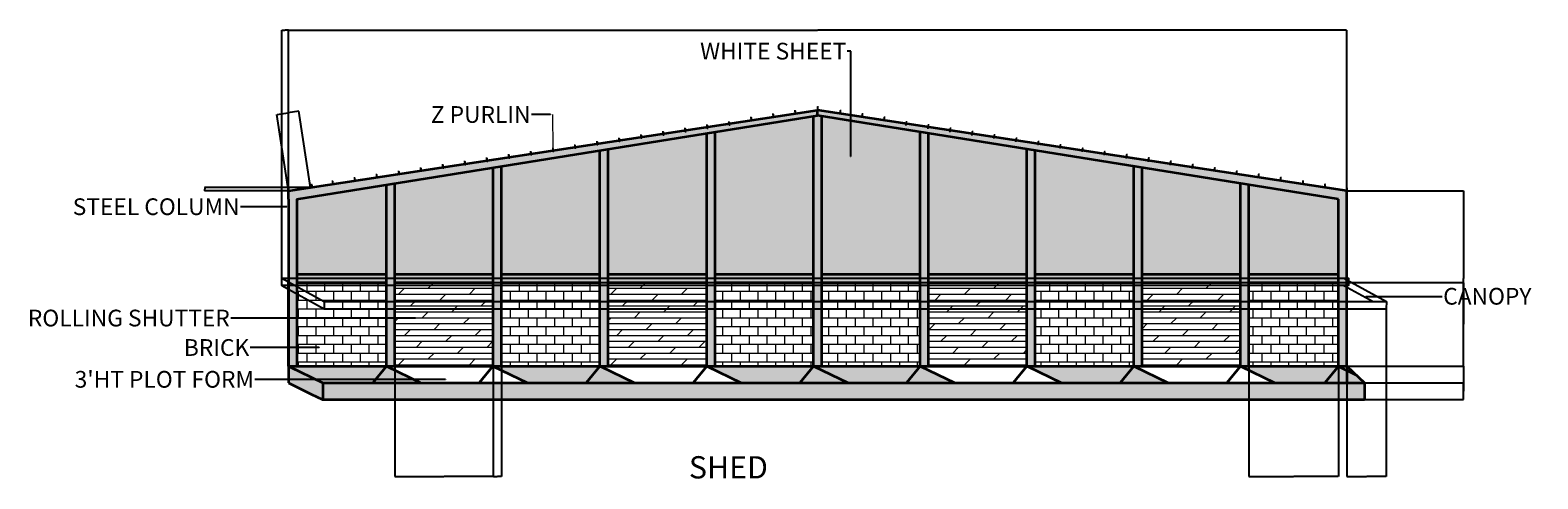
# Model space of a CAD drawing. Units: inches. Extents: x 1136 to 4385, y 1177 to 2144.
import ezdxf
from ezdxf import colors
from ezdxf.entities.mleader import LeaderData, LeaderLine
from ezdxf.math import Vec2, Vec3

# ---------------------------------------------------------------- set-up
doc = ezdxf.new("R2010")
doc.units = ezdxf.units.IN
for name, color, linetype, lineweight in [('A-ANNO-DIMS', 2, 'Continuous', 18), ('A-ANNO-TEXT', 7, 'Continuous', 18), ('A-DOOR-PATT', 8, 'Continuous', 13), ('A-FLOR-PLAT', 7, 'Continuous', 35), ('A-WALL-PATT', 8, 'Continuous', 13), ('S-BEAM', 7, 'Continuous', 35), ('S-COLS', 7, 'Continuous', 35), ('S-ROOF-PURL', 7, 'Continuous', 25)]:
    doc.layers.add(name, color=color, linetype=linetype, lineweight=lineweight)
for name, color, linetype, lineweight, true_color in [('A-FLOR-PATT', 30, 'Continuous', 13, 0xf26722), ('A-ROOF-CNPY', 240, 'Continuous', 25, 0xed1f24), ('A-WALL-CLAD-PATT', 7, 'Continuous', 13, 0xffffff), ('S-FRAM-PATT', 252, 'Continuous', 13, 0x939598)]:
    doc.layers.add(name, color=color, linetype=linetype, lineweight=lineweight, true_color=true_color)
doc.styles.get("Standard").update_dxf_attribs({"font": 'arial.ttf'})
doc.dimstyles.get("Standard").update_dxf_attribs({"dimtxt": 0.18, "dimasz": 0.18, "dimexe": 0.18, "dimexo": 0.0625, "dimgap": 0.09, "dimtad": 0, "dimtih": 1, "dimtoh": 1, "dimdec": 4, "dimzin": 0, "dimdsep": 46, "dimtxsty": 'Standard', "dimcen": 0.09, "dimadec": 0, "dimazin": 0, "dimtfac": 1, "dimtdec": 4, "dimtofl": 0, "dimtmove": 0, "dimatfit": 3, "dimfxl": 1, "dimtolj": 1, "dimtzin": 0, "dimarcsym": 0})

# ---------------------------------------------------------------- blocks, each defined once
blk = doc.blocks.new('PURLIN-Z-6IN')
blk.add_lwpolyline([(0, 6), (2, 6), (2, 0), (4, 0)])
blk = doc.blocks.new('*D2')
at = {"layer": 'A-ANNO-DIMS', "color": 0, "lineweight": -2, "transparency": 16777216}
for p, q in [((1742.7, 1810.9), (1743.7, 1810.9)), ((1742.7, 1804.9), (1743.7, 1804.9)), ((1743.5, 1810.7), (1743.5, 1808.1)), ((1743.5, 1805.1), (1743.5, 1807.7))]:
    blk.add_line(p, q, dxfattribs=at)
at = {"layer": 'A-ANNO-DIMS', "color": 0, "transparency": 16777216}
for points in [[(1743.5, 1810.7), (1743.6, 1810.7), (1743.5, 1810.9)], [(1743.5, 1805.1), (1743.6, 1805.1), (1743.5, 1804.9)]]:
    blk.add_solid(points, dxfattribs=at)
at = {"layer": 'Defpoints', "color": 0, "transparency": 16777216}
for p in [(1742.6, 1810.9), (1742.6, 1804.9), (1743.5, 1810.9)]:
    blk.add_point(p, dxfattribs=at)
at = {"layer": 'A-ANNO-DIMS', "color": 0, "transparency": 16777216, "insert": (1743.5, 1807.9), "char_height": 0.18, "attachment_point": 5}
blk.add_mtext('\\A1;Z PURLIN 6 TYP.', dxfattribs=at)
blk = doc.blocks.new('*D3')
at = {"layer": 'A-ANNO-DIMS', "color": 0, "lineweight": -2, "transparency": 16777216}
for p, q in [((1738.6, 1804.8), (1738.6, 1803.8)), ((1738.8, 1804), (1740.2, 1804)), ((1742.5, 1804), (1741.1, 1804)), ((1742.6, 1804.8), (1742.6, 1803.8))]:
    blk.add_line(p, q, dxfattribs=at)
at = {"layer": 'A-ANNO-DIMS', "color": 0, "transparency": 16777216}
for points in [[(1738.8, 1804), (1738.8, 1804), (1738.6, 1804)], [(1742.5, 1804), (1742.5, 1804), (1742.6, 1804)]]:
    blk.add_solid(points, dxfattribs=at)
at = {"layer": 'Defpoints', "color": 0, "transparency": 16777216}
for p in [(1738.6, 1804.9), (1742.6, 1804.9), (1742.6, 1804)]:
    blk.add_point(p, dxfattribs=at)
at = {"layer": 'A-ANNO-DIMS', "color": 0, "transparency": 16777216, "insert": (1740.6, 1804), "char_height": 0.18, "attachment_point": 5}
blk.add_mtext('\\A1;4 TYP.', dxfattribs=at)
blk = doc.blocks.new('*D4')
at = {"layer": 'A-ANNO-DIMS', "color": 0, "lineweight": -2, "transparency": 16777216}
for p, q in [((1693.184241, 1797.715563), (1693.184241, 2143.833063)), ((1693.364241, 2143.653063), (2832.824241, 2143.653063)), ((3973.004241, 2143.653063), (2833.544241, 2143.653063)), ((3973.184241, 1797.715563), (3973.184241, 2143.833063))]:
    blk.add_line(p, q, dxfattribs=at)
at = {"layer": 'A-ANNO-DIMS', "color": 0, "transparency": 16777216}
for points in [[(1693.364241, 2143.683063), (1693.364241, 2143.623063), (1693.184241, 2143.653063)], [(3973.004241, 2143.683063), (3973.004241, 2143.623063), (3973.184241, 2143.653063)]]:
    blk.add_solid(points, dxfattribs=at)
at = {"layer": 'Defpoints', "color": 0, "transparency": 16777216}
for p in [(3973.184241, 2143.653063), (1693.184241, 1797.653063), (3973.184241, 1797.653063)]:
    blk.add_point(p, dxfattribs=at)
at = {"layer": 'A-ANNO-DIMS', "color": 0, "transparency": 16777216, "insert": (2833.184241, 2143.653063), "char_height": 0.18, "attachment_point": 5}
blk.add_mtext('\\A1;2280', dxfattribs=at)
blk = doc.blocks.new('*D5')
at = {"layer": 'A-ANNO-DIMS', "color": 0, "lineweight": -2, "transparency": 16777216}
for p, q in [((3973.2, 1797.7), (4224.9, 1797.7)), ((4224.7, 1797.5), (4224.7, 1608.8)), ((4224.7, 1419.8), (4224.7, 1608.5)), ((3973.2, 1419.7), (4224.9, 1419.7))]:
    blk.add_line(p, q, dxfattribs=at)
at = {"layer": 'A-ANNO-DIMS', "color": 0, "transparency": 16777216}
for points in [[(4224.7, 1797.5), (4224.8, 1797.5), (4224.7, 1797.7)], [(4224.7, 1419.8), (4224.8, 1419.8), (4224.7, 1419.7)]]:
    blk.add_solid(points, dxfattribs=at)
at = {"layer": 'Defpoints', "color": 0, "transparency": 16777216}
for p in [(3973.2, 1797.7), (4224.7, 1797.7), (3973.2, 1419.7)]:
    blk.add_point(p, dxfattribs=at)
at = {"layer": 'A-ANNO-DIMS', "color": 0, "transparency": 16777216, "insert": (4224.7, 1608.7), "char_height": 0.18, "attachment_point": 5}
blk.add_mtext('\\A1;378', dxfattribs=at)
blk = doc.blocks.new('*D6')
at = {"layer": 'A-ANNO-DIMS', "color": 0, "lineweight": -2, "transparency": 16777216}
for p, q in [((4058.5, 1543.4), (4058.5, 1181.5)), ((3973.2, 1419.6), (3973.2, 1181.5)), ((3973.4, 1181.7), (4015.5, 1181.7)), ((4058.3, 1181.7), (4016.2, 1181.7))]:
    blk.add_line(p, q, dxfattribs=at)
at = {"layer": 'A-ANNO-DIMS', "color": 0, "transparency": 16777216}
for points in [[(3973.4, 1181.7), (3973.4, 1181.6), (3973.2, 1181.7)], [(4058.3, 1181.7), (4058.3, 1181.6), (4058.5, 1181.7)]]:
    blk.add_solid(points, dxfattribs=at)
at = {"layer": 'Defpoints', "color": 0, "transparency": 16777216}
for p in [(4058.5, 1543.5), (3973.2, 1419.7), (3973.2, 1181.7)]:
    blk.add_point(p, dxfattribs=at)
at = {"layer": 'A-ANNO-DIMS', "color": 0, "transparency": 16777216, "insert": (4015.8, 1181.7), "char_height": 0.18, "attachment_point": 5}
blk.add_mtext('\\A1;85.3', dxfattribs=at)
blk = doc.blocks.new('*D7')
at = {"layer": 'A-ANNO-DIMS', "color": 0, "lineweight": -2, "transparency": 16777216}
for p, q in [((1678.6, 1609.2), (1678.6, 2143.8)), ((1678.8, 2143.7), (1685.5, 2143.7)), ((1693, 2143.7), (1686.2, 2143.7)), ((1693.2, 1797.7), (1693.2, 2143.8))]:
    blk.add_line(p, q, dxfattribs=at)
at = {"layer": 'A-ANNO-DIMS', "color": 0, "transparency": 16777216}
for points in [[(1678.8, 2143.7), (1678.8, 2143.6), (1678.6, 2143.7)], [(1693, 2143.7), (1693, 2143.6), (1693.2, 2143.7)]]:
    blk.add_solid(points, dxfattribs=at)
at = {"layer": 'Defpoints', "color": 0, "transparency": 16777216}
for p in [(1693.2, 2143.7), (1693.2, 1797.7), (1678.6, 1609.1)]:
    blk.add_point(p, dxfattribs=at)
at = {"layer": 'A-ANNO-DIMS', "color": 0, "transparency": 16777216, "insert": (1685.9, 2143.7), "char_height": 0.18, "attachment_point": 5}
blk.add_mtext('\\A1;14.61', dxfattribs=at)
blk = doc.blocks.new('*D8')
at = {"layer": 'A-ANNO-DIMS', "color": 0, "lineweight": -2, "transparency": 16777216}
for p, q in [((4011.4, 1383.7), (4224.9, 1383.7)), ((4224.7, 1383.5), (4224.7, 1365.8)), ((4224.7, 1347.8), (4224.7, 1365.5)), ((4011.4, 1347.7), (4224.9, 1347.7))]:
    blk.add_line(p, q, dxfattribs=at)
at = {"layer": 'A-ANNO-DIMS', "color": 0, "transparency": 16777216}
for points in [[(4224.7, 1383.5), (4224.8, 1383.5), (4224.7, 1383.7)], [(4224.7, 1347.8), (4224.8, 1347.8), (4224.7, 1347.7)]]:
    blk.add_solid(points, dxfattribs=at)
at = {"layer": 'Defpoints', "color": 0, "transparency": 16777216}
for p in [(4011.3, 1383.7), (4224.7, 1383.7), (4011.3, 1347.7)]:
    blk.add_point(p, dxfattribs=at)
at = {"layer": 'A-ANNO-DIMS', "color": 0, "transparency": 16777216, "insert": (4224.7, 1365.7), "char_height": 0.18, "attachment_point": 5}
blk.add_mtext('\\A1;36', dxfattribs=at)
blk = doc.blocks.new('*D9')
at = {"layer": 'A-ANNO-DIMS', "color": 0, "lineweight": -2, "transparency": 16777216}
for p, q in [((1922.2, 1599.7), (4224.9, 1599.7)), ((4224.7, 1599.5), (4224.7, 1509.8)), ((4224.7, 1419.8), (4224.7, 1509.5)), ((1922.2, 1419.7), (4224.9, 1419.7))]:
    blk.add_line(p, q, dxfattribs=at)
at = {"layer": 'A-ANNO-DIMS', "color": 0, "transparency": 16777216}
for points in [[(4224.7, 1599.5), (4224.8, 1599.5), (4224.7, 1599.7)], [(4224.7, 1419.8), (4224.8, 1419.8), (4224.7, 1419.7)]]:
    blk.add_solid(points, dxfattribs=at)
at = {"layer": 'Defpoints', "color": 0, "transparency": 16777216}
for p in [(1922.2, 1599.7), (4224.7, 1599.7), (1922.2, 1419.7)]:
    blk.add_point(p, dxfattribs=at)
at = {"layer": 'A-ANNO-DIMS', "color": 0, "transparency": 16777216, "insert": (4224.7, 1509.7), "char_height": 0.18, "attachment_point": 5}
blk.add_mtext('\\A1;180', dxfattribs=at)
blk = doc.blocks.new('*D10')
at = {"layer": 'A-ANNO-DIMS', "color": 0, "lineweight": -2, "transparency": 16777216}
for p, q in [((1922.2, 1419.6), (1922.2, 1181.5)), ((2134.2, 1419.6), (2134.2, 1181.5)), ((1922.4, 1181.7), (2027.9, 1181.7)), ((2134, 1181.7), (2028.5, 1181.7))]:
    blk.add_line(p, q, dxfattribs=at)
at = {"layer": 'A-ANNO-DIMS', "color": 0, "transparency": 16777216}
for points in [[(1922.4, 1181.7), (1922.4, 1181.6), (1922.2, 1181.7)], [(2134, 1181.7), (2134, 1181.6), (2134.2, 1181.7)]]:
    blk.add_solid(points, dxfattribs=at)
at = {"layer": 'Defpoints', "color": 0, "transparency": 16777216}
for p in [(1922.2, 1419.7), (2134.2, 1419.7), (2134.2, 1181.7)]:
    blk.add_point(p, dxfattribs=at)
at = {"layer": 'A-ANNO-DIMS', "color": 0, "transparency": 16777216, "insert": (2028.2, 1181.7), "char_height": 0.18, "attachment_point": 5}
blk.add_mtext('\\A1;212', dxfattribs=at)
blk = doc.blocks.new('*D11')
at = {"layer": 'A-ANNO-DIMS', "color": 0, "lineweight": -2, "transparency": 16777216}
for p, q in [((2134.2, 1419.6), (2134.2, 1181.5)), ((2152.2, 1419.6), (2152.2, 1181.5)), ((2134.4, 1181.7), (2143, 1181.7)), ((2152, 1181.7), (2143.4, 1181.7))]:
    blk.add_line(p, q, dxfattribs=at)
at = {"layer": 'A-ANNO-DIMS', "color": 0, "transparency": 16777216}
for points in [[(2134.4, 1181.7), (2134.4, 1181.6), (2134.2, 1181.7)], [(2152, 1181.7), (2152, 1181.6), (2152.2, 1181.7)]]:
    blk.add_solid(points, dxfattribs=at)
at = {"layer": 'Defpoints', "color": 0, "transparency": 16777216}
for p in [(2134.2, 1419.7), (2152.2, 1419.7), (2152.2, 1181.7)]:
    blk.add_point(p, dxfattribs=at)
at = {"layer": 'A-ANNO-DIMS', "color": 0, "transparency": 16777216, "insert": (2143.2, 1181.7), "char_height": 0.18, "attachment_point": 5}
blk.add_mtext('\\A1;18', dxfattribs=at)
blk = doc.blocks.new('*D12')
at = {"layer": 'A-ANNO-DIMS', "color": 0, "lineweight": -2, "transparency": 16777216}
for p, q in [((3762.2, 1419.6), (3762.2, 1181.5)), ((3955.2, 1419.6), (3955.2, 1181.5)), ((3762.4, 1181.7), (3858.4, 1181.7)), ((3955, 1181.7), (3859, 1181.7))]:
    blk.add_line(p, q, dxfattribs=at)
at = {"layer": 'A-ANNO-DIMS', "color": 0, "transparency": 16777216}
for points in [[(3762.4, 1181.7), (3762.4, 1181.6), (3762.2, 1181.7)], [(3955, 1181.7), (3955, 1181.6), (3955.2, 1181.7)]]:
    blk.add_solid(points, dxfattribs=at)
at = {"layer": 'Defpoints', "color": 0, "transparency": 16777216}
for p in [(3762.2, 1419.7), (3955.2, 1419.7), (3955.2, 1181.7)]:
    blk.add_point(p, dxfattribs=at)
at = {"layer": 'A-ANNO-DIMS', "color": 0, "transparency": 16777216, "insert": (3858.7, 1181.7), "char_height": 0.18, "attachment_point": 5}
blk.add_mtext('\\A1;193', dxfattribs=at)
blk = doc.blocks.new('*D13')
at = {"layer": 'A-ANNO-DIMS', "color": 0, "lineweight": -2, "transparency": 16777216}
for p, q in [((1693.2, 1797.7), (1668.1, 1961.9)), ((1668.3, 1961.8), (1691.6, 1965.3)), ((1715.4, 1969), (1692.1, 1965.4)), ((1740.6, 1805), (1715.6, 1969.2))]:
    blk.add_line(p, q, dxfattribs=at)
at = {"layer": 'A-ANNO-DIMS', "color": 0, "transparency": 16777216}
for points in [[(1668.3, 1961.8), (1668.3, 1961.8), (1668.1, 1961.8)], [(1715.4, 1969), (1715.4, 1968.9), (1715.6, 1969)]]:
    blk.add_solid(points, dxfattribs=at)
at = {"layer": 'Defpoints', "color": 0, "transparency": 16777216}
for p in [(1715.6, 1969), (1693.2, 1797.7), (1740.6, 1804.9)]:
    blk.add_point(p, dxfattribs=at)
at = {"layer": 'A-ANNO-DIMS', "color": 0, "transparency": 16777216, "insert": (1691.9, 1965.4), "char_height": 0.18, "attachment_point": 5}
blk.add_mtext('\\A1;48', dxfattribs=at)
blk = doc.blocks.new('*D14')
at = {"layer": 'A-ANNO-DIMS', "color": 0, "lineweight": -2, "transparency": 16777216}
for p, q in [((1740.6, 1804.9), (1512.4, 1804.9)), ((1693.1, 1797.7), (1512.4, 1797.7)), ((1512.6, 1804.7), (1512.6, 1801.5)), ((1512.6, 1797.8), (1512.6, 1801.1))]:
    blk.add_line(p, q, dxfattribs=at)
at = {"layer": 'A-ANNO-DIMS', "color": 0, "transparency": 16777216}
for points in [[(1512.5, 1804.7), (1512.6, 1804.7), (1512.6, 1804.9)], [(1512.5, 1797.8), (1512.6, 1797.8), (1512.6, 1797.7)]]:
    blk.add_solid(points, dxfattribs=at)
at = {"layer": 'Defpoints', "color": 0, "transparency": 16777216}
for p in [(1512.6, 1804.9), (1693.2, 1797.7), (1740.6, 1804.9)]:
    blk.add_point(p, dxfattribs=at)
at = {"layer": 'A-ANNO-DIMS', "color": 0, "transparency": 16777216, "insert": (1512.6, 1801.3), "char_height": 0.18, "attachment_point": 5}
blk.add_mtext('\\A1;7.242', dxfattribs=at)
blk = doc.blocks.new('*D15')
at = {"layer": 'A-ANNO-DIMS', "color": 0, "lineweight": -2, "transparency": 16777216}
for p, q in [((3973.2, 1419.7), (4224.9, 1419.7)), ((4224.7, 1419.5), (4224.7, 1383.8)), ((4224.7, 1347.8), (4224.7, 1383.5)), ((4011.4, 1347.7), (4224.9, 1347.7))]:
    blk.add_line(p, q, dxfattribs=at)
at = {"layer": 'A-ANNO-DIMS', "color": 0, "transparency": 16777216}
for points in [[(4224.7, 1419.5), (4224.8, 1419.5), (4224.7, 1419.7)], [(4224.7, 1347.8), (4224.8, 1347.8), (4224.7, 1347.7)]]:
    blk.add_solid(points, dxfattribs=at)
at = {"layer": 'Defpoints', "color": 0, "transparency": 16777216}
for p in [(3973.2, 1419.7), (4011.3, 1347.7), (4224.7, 1347.7)]:
    blk.add_point(p, dxfattribs=at)
at = {"layer": 'A-ANNO-DIMS', "color": 0, "transparency": 16777216, "insert": (4224.7, 1383.7), "char_height": 0.18, "attachment_point": 5}
blk.add_mtext('\\A1;72', dxfattribs=at)

msp = doc.modelspace()

# ---------------------------------------------------------------- hatches: boundary and pattern name
at = {"layer": 'A-DOOR-PATT'}
h = msp.add_hatch(dxfattribs=at)
h.set_pattern_fill('DOLMIT', color=256, scale=2)
h.paths.add_polyline_path([(2134.1842, 1599.6531), (1922.1842, 1599.6531), (1922.1842, 1419.6531), (2134.1842, 1419.6531)])
h.paths.add_polyline_path([(2594.1842, 1599.6531), (2382.1842, 1599.6531), (2382.1842, 1419.6531), (2594.1842, 1419.6531)])
h.paths.add_polyline_path([(3284.1842, 1599.6531), (3072.1842, 1599.6531), (3072.1842, 1419.6531), (3284.1842, 1419.6531)])
h.paths.add_polyline_path([(3744.1842, 1599.6531), (3532.1842, 1599.6531), (3532.1842, 1419.6531), (3744.1842, 1419.6531)])
at = {"layer": 'A-FLOR-PATT'}
h = msp.add_hatch(color=256, dxfattribs=at)
h.dxf.hatch_style = 1
h.paths.add_polyline_path([(1904.1842, 1419.6531), (1693.1842, 1419.6531), (1767.3542, 1383.6531), (1874.7817, 1383.6531)])
h.paths.add_polyline_path([(4011.303, 1383.6531), (1767.3542, 1383.6531), (1767.3542, 1347.6531), (4011.303, 1347.6531)])
h.paths.add_polyline_path([(1767.3542, 1383.6531), (1693.1842, 1419.6531), (1693.1842, 1383.6531), (1742.1622, 1359.5845), (1766.442, 1347.6531), (1767.3542, 1347.6531)])
h.paths.add_polyline_path([(3992.81, 1401.1182), (3973.1842, 1410.644), (3973.1842, 1383.6531), (4011.303, 1383.6531)])
h.paths.add_polyline_path([(3973.1842, 1419.6531), (3955.5362, 1419.6531), (3955.277, 1419.3357), (3992.81, 1401.1182)])
h.paths.add_polyline_path([(3973.1842, 1410.644), (3955.277, 1419.3357), (3926.1337, 1383.6531), (3973.1842, 1383.6531)])
h.paths.add_polyline_path([(3955.1842, 1419.2221), (3955.1842, 1419.3807), (3954.6231, 1419.6531), (3744.4245, 1419.6531), (3818.5945, 1383.6531), (3926.1337, 1383.6531)])
h.paths.add_polyline_path([(3514.4245, 1419.6531), (3514.1842, 1419.6531), (3484.7817, 1383.6531), (3588.5945, 1383.6531)])
h.paths.add_polyline_path([(3514.1842, 1419.6531), (3284.4245, 1419.6531), (3358.5945, 1383.6531), (3484.7817, 1383.6531)])
h.paths.add_polyline_path([(3054.4245, 1419.6531), (3054.1842, 1419.6531), (3024.7817, 1383.6531), (3128.5945, 1383.6531)])
h.paths.add_polyline_path([(3054.1842, 1419.6531), (2824.4245, 1419.6531), (2898.5945, 1383.6531), (3024.7817, 1383.6531)])
h.paths.add_polyline_path([(2824.4245, 1419.6531), (2824.1842, 1419.6531), (2794.7817, 1383.6531), (2898.5945, 1383.6531)])
h.paths.add_polyline_path([(2364.1842, 1419.6531), (2133.5344, 1419.6531), (2207.7043, 1383.6531), (2334.7817, 1383.6531)])
h.paths.add_polyline_path([(2364.4245, 1419.6531), (2364.1842, 1419.6531), (2334.7817, 1383.6531), (2438.5945, 1383.6531)])
h.paths.add_polyline_path([(2824.1842, 1419.6531), (2594.4245, 1419.6531), (2668.5945, 1383.6531), (2794.7817, 1383.6531)])
h.paths.add_polyline_path([(1904.1842, 1419.6531), (1874.7817, 1383.6531), (1978.3542, 1383.6531)])
at = {"layer": 'A-WALL-CLAD-PATT'}
h = msp.add_hatch(color=256, dxfattribs=at)
h.dxf.hatch_style = 1
h.paths.add_polyline_path([(1904.1842, 1810.6156), (1711.1842, 1779.6531), (1711.1842, 1617.6531), (1904.1842, 1617.6531)])
h.paths.add_polyline_path([(2134.1842, 1847.514), (1922.1842, 1813.5033), (1922.1842, 1617.6531), (2134.1842, 1617.6531)])
h.paths.add_polyline_path([(2364.1842, 1884.4124), (2152.1842, 1850.4017), (2152.1842, 1617.6531), (2364.1842, 1617.6531)])
h.paths.add_polyline_path([(2594.1842, 1921.3108), (2382.1842, 1887.3001), (2382.1842, 1617.6531), (2594.1842, 1617.6531)])
h.paths.add_polyline_path([(2824.1842, 1958.2092), (2612.1842, 1924.1985), (2612.1842, 1617.6531), (2824.1842, 1617.6531)])
h.paths.add_polyline_path([(3054.1842, 1924.1985), (2842.1842, 1958.2092), (2842.1842, 1617.6531), (3054.1842, 1617.6531)])
h.paths.add_polyline_path([(3284.1842, 1887.3001), (3072.1842, 1921.3108), (3072.1842, 1617.6531), (3284.1842, 1617.6531)])
h.paths.add_polyline_path([(3514.1842, 1850.4017), (3302.1842, 1884.4124), (3302.1842, 1617.6531), (3514.1842, 1617.6531)])
h.paths.add_polyline_path([(3744.1842, 1813.5033), (3532.1842, 1847.514), (3532.1842, 1617.6531), (3744.1842, 1617.6531)])
h.paths.add_polyline_path([(3955.1842, 1779.6531), (3762.1842, 1810.6156), (3762.1842, 1617.6531), (3955.1842, 1617.6531)])
at = {"layer": 'A-WALL-PATT'}
h = msp.add_hatch(dxfattribs=at)
h.set_pattern_fill('BRICK', color=256, scale=3)
h.paths.add_polyline_path([(1904.1842, 1599.6531), (1711.1842, 1599.6531), (1711.1842, 1419.6531), (1904.1842, 1419.6531)])
h.paths.add_polyline_path([(2364.1842, 1599.6531), (2152.1842, 1599.6531), (2152.1842, 1419.6531), (2364.1842, 1419.6531)])
h.paths.add_polyline_path([(2824.1842, 1599.6531), (2612.1842, 1599.6531), (2612.1842, 1419.6531), (2824.1842, 1419.6531)])
h.paths.add_polyline_path([(3054.1842, 1599.6531), (2842.1842, 1599.6531), (2842.1842, 1419.6531), (3054.1842, 1419.6531)])
h.paths.add_polyline_path([(3514.1842, 1599.6531), (3302.1842, 1599.6531), (3302.1842, 1419.6531), (3514.1842, 1419.6531)])
h.paths.add_polyline_path([(3955.1842, 1599.6531), (3762.1842, 1599.6531), (3762.1842, 1419.6531), (3955.1842, 1419.6531)])
at = {"layer": 'S-FRAM-PATT'}
h = msp.add_hatch(color=256, dxfattribs=at)
h.dxf.hatch_style = 1
h.paths.add_polyline_path([(1711.1842, 1779.6531), (2833.1842, 1959.6531), (2833.1842, 1971.6531), (1693.1842, 1797.6531), (1693.1842, 1779.6531), (1693.1842, 1419.6531), (1711.1842, 1419.6531)])
h.paths.add_polyline_path([(1904.1842, 1617.6531), (1711.1842, 1617.6531), (1711.1842, 1599.6531), (1904.1842, 1599.6531)], flags=17)
h.paths.add_polyline_path([(2134.1842, 1617.6531), (1922.1842, 1617.6531), (1922.1842, 1599.6531), (2134.1842, 1599.6531)], flags=17)
h = msp.add_hatch(color=256, dxfattribs=at)
h.dxf.hatch_style = 1
h.paths.add_polyline_path([(1922.1842, 1813.5033), (1904.1842, 1810.6156), (1904.1842, 1419.6531), (1922.1842, 1419.6531)])
h.paths.add_polyline_path([(2152.1842, 1850.4017), (2134.1842, 1847.514), (2134.1842, 1419.6531), (2152.1842, 1419.6531)])
h.paths.add_polyline_path([(2382.1842, 1887.3001), (2364.1842, 1884.4124), (2364.1842, 1419.6531), (2382.1842, 1419.6531)])
h.paths.add_polyline_path([(2364.1842, 1617.6531), (2152.1842, 1617.6531), (2152.1842, 1599.6531), (2364.1842, 1599.6531)])
h.paths.add_polyline_path([(2594.1842, 1617.6531), (2382.1842, 1617.6531), (2382.1842, 1599.6531), (2594.1842, 1599.6531)])
h.paths.add_polyline_path([(2612.1842, 1924.1985), (2594.1842, 1921.3108), (2594.1842, 1419.6531), (2612.1842, 1419.6531)])
h.paths.add_polyline_path([(2824.1842, 1617.6531), (2612.1842, 1617.6531), (2612.1842, 1599.6531), (2824.1842, 1599.6531)])
h.paths.add_polyline_path([(2842.1842, 1958.2092), (2833.1842, 1959.6531), (2824.1842, 1958.2092), (2824.1842, 1419.6531), (2842.1842, 1419.6531)])
h.paths.add_polyline_path([(3054.1842, 1617.6531), (2842.1842, 1617.6531), (2842.1842, 1599.6531), (3054.1842, 1599.6531)], flags=17)
h.paths.add_polyline_path([(3072.1842, 1921.3108), (3054.1842, 1924.1985), (3054.1842, 1419.6531), (3072.1842, 1419.6531)], flags=17)
h.paths.add_polyline_path([(3284.1842, 1617.6531), (3072.1842, 1617.6531), (3072.1842, 1599.6531), (3284.1842, 1599.6531)], flags=17)
h.paths.add_polyline_path([(3302.1842, 1884.4124), (3284.1842, 1887.3001), (3284.1842, 1419.6531), (3302.1842, 1419.6531)], flags=17)
h.paths.add_polyline_path([(3514.1842, 1617.6531), (3302.1842, 1617.6531), (3302.1842, 1599.6531), (3514.1842, 1599.6531)], flags=17)
h.paths.add_polyline_path([(3532.1842, 1847.514), (3514.1842, 1850.4017), (3514.1842, 1419.6531), (3532.1842, 1419.6531)], flags=17)
h.paths.add_polyline_path([(3955.1842, 1617.6531), (3762.1842, 1617.6531), (3762.1842, 1599.6531), (3955.1842, 1599.6531)], flags=17)
h.paths.add_polyline_path([(3973.1842, 1797.6531), (2833.1842, 1971.6531), (2833.1842, 1959.6531), (2842.1842, 1958.2092), (3955.1842, 1779.6531), (3955.1842, 1419.6531), (3973.1842, 1419.6531)])
h = msp.add_hatch(color=256, dxfattribs=at)
h.dxf.hatch_style = 1
h.paths.add_polyline_path([(3762.1842, 1810.6156), (3744.1842, 1813.5033), (3744.1842, 1419.6531), (3762.1842, 1419.6531)])
h.paths.add_polyline_path([(3744.1842, 1617.6531), (3532.1842, 1617.6531), (3532.1842, 1599.6531), (3744.1842, 1599.6531)])

# ---------------------------------------------------------------- linework, layer by layer
at = {"layer": 'A-ANNO-TEXT'}
msp.add_line((2261.8285, 1961.7238), (2262.8285, 1888.9845), dxfattribs=at)
at = {"layer": 'A-FLOR-PLAT'}
for p, q in [((1693.1842, 1419.6531), (3973.1842, 1419.6531)), ((1693.1842, 1419.6531), (1693.1842, 1383.6531)), ((1693.1842, 1419.6531), (1767.3542, 1383.6531)), ((1693.1842, 1419.6531), (1725.6025, 1403.9987)), ((1904.1842, 1419.6531), (1874.7817, 1383.6531)), ((1904.1842, 1419.6531), (1978.3542, 1383.6531)), ((2133.5344, 1419.6531), (2104.1318, 1383.6531)), ((2133.5344, 1419.6531), (2207.7043, 1383.6531)), ((2364.1842, 1419.6531), (2334.7817, 1383.6531)), ((2364.4245, 1419.6531), (2438.5945, 1383.6531)), ((2594.1842, 1419.6531), (2564.7817, 1383.6531)), ((2594.4245, 1419.6531), (2668.5945, 1383.6531)), ((2824.1842, 1419.6531), (2794.7817, 1383.6531)), ((2824.4245, 1419.6531), (2898.5945, 1383.6531)), ((3054.1842, 1419.6531), (3024.7817, 1383.6531)), ((3054.4245, 1419.6531), (3128.5945, 1383.6531)), ((3284.1842, 1419.6531), (3254.7817, 1383.6531)), ((3284.4245, 1419.6531), (3358.5945, 1383.6531)), ((3514.1842, 1419.6531), (3484.7817, 1383.6531)), ((3514.4245, 1419.6531), (3588.5945, 1383.6531)), ((3744.1842, 1419.6531), (3714.7817, 1383.6531)), ((3744.4245, 1419.6531), (3818.5945, 1383.6531)), ((3955.5362, 1419.6531), (3926.1337, 1383.6531)), ((3954.6231, 1419.6531), (3992.81, 1401.1182)), ((3973.1842, 1419.6531), (4011.303, 1383.6531)), ((3973.1842, 1410.644), (3973.1842, 1383.6531)), ((1693.1842, 1383.6531), (1742.1622, 1359.5845)), ((1767.3542, 1383.6531), (4011.303, 1383.6531)), ((1767.3542, 1383.6531), (1767.3542, 1347.6531)), ((4011.303, 1383.6531), (4011.303, 1347.6531)), ((1742.1622, 1359.5845), (1766.442, 1347.6531)), ((1766.442, 1347.6531), (4011.303, 1347.6531))]:
    msp.add_line(p, q, dxfattribs=at)
at = {"layer": 'A-ROOF-CNPY'}
for p, q in [((1678.5734, 1609.1255), (1770.081, 1559.1366)), ((1678.5734, 1593.4739), (1770.0695, 1543.4913)), ((3967.2276, 1609.1255), (4058.7352, 1559.1366)), ((3967.2276, 1593.4739), (4030.084, 1559.1366)), ((1770.0695, 1543.4913), (4058.4842, 1543.4913)), ((1770.081, 1559.1366), (4058.7352, 1559.1366)), ((1770.081, 1559.1366), (1770.081, 1543.4913)), ((4058.7352, 1559.1366), (4058.4842, 1543.4913))]:
    msp.add_line(p, q, dxfattribs=at)
msp.add_lwpolyline([(1678.5734, 1609.1255), (3977.0566, 1609.1255), (3977.0566, 1593.4739), (1678.5734, 1593.4739)], close=True, dxfattribs=at)
at = {"layer": 'S-BEAM'}
for p, q in [((1693.1842, 1797.6531), (2833.1842, 1971.6531)), ((1711.1842, 1779.6531), (2833.1842, 1959.6531)), ((2833.1842, 1959.6531), (2833.1842, 1971.6531)), ((3973.1842, 1797.6531), (2833.1842, 1971.6531)), ((2833.1842, 1959.6531), (2833.1842, 1971.6531)), ((3955.1842, 1779.6531), (2833.1842, 1959.6531)), ((1693.1842, 1779.6531), (1693.1842, 1797.6531)), ((1711.1842, 1617.6531), (1904.1842, 1617.6531)), ((1711.1842, 1599.6531), (1904.1842, 1599.6531)), ((1922.1842, 1617.6531), (2134.1842, 1617.6531)), ((1922.1842, 1599.6531), (2134.1842, 1599.6531)), ((2152.1842, 1617.6531), (2364.1842, 1617.6531)), ((2152.1842, 1599.6531), (2364.1842, 1599.6531)), ((2382.1842, 1617.6531), (2594.1842, 1617.6531)), ((2382.1842, 1599.6531), (2594.1842, 1599.6531)), ((2612.1842, 1617.6531), (2824.1842, 1617.6531)), ((2612.1842, 1599.6531), (2824.1842, 1599.6531)), ((2842.1842, 1617.6531), (3054.1842, 1617.6531)), ((2842.1842, 1599.6531), (3054.1842, 1599.6531)), ((3072.1842, 1617.6531), (3284.1842, 1617.6531)), ((3072.1842, 1599.6531), (3284.1842, 1599.6531)), ((3302.1842, 1617.6531), (3514.1842, 1617.6531)), ((3302.1842, 1599.6531), (3514.1842, 1599.6531)), ((3532.1842, 1617.6531), (3744.1842, 1617.6531)), ((3532.1842, 1599.6531), (3744.1842, 1599.6531)), ((3762.1842, 1617.6531), (3955.1842, 1617.6531)), ((3762.1842, 1599.6531), (3955.1842, 1599.6531))]:
    msp.add_line(p, q, dxfattribs=at)
at = {"layer": 'S-COLS'}
for p, q in [((2824.1842, 1419.6531), (2824.1842, 1958.2092)), ((2842.1842, 1419.6531), (2842.1842, 1958.2092)), ((2594.1842, 1419.6531), (2594.1842, 1921.3108)), ((2612.1842, 1419.6531), (2612.1842, 1924.1985)), ((3054.1842, 1419.6531), (3054.1842, 1924.1985)), ((3072.1842, 1419.6531), (3072.1842, 1921.3108)), ((2364.1842, 1419.6531), (2364.1842, 1884.4124)), ((2382.1842, 1419.6531), (2382.1842, 1887.3001)), ((3284.1842, 1419.6531), (3284.1842, 1887.3001)), ((3302.1842, 1419.6531), (3302.1842, 1884.4124)), ((2134.1842, 1419.6531), (2134.1842, 1847.514)), ((2152.1842, 1419.6531), (2152.1842, 1850.4017)), ((3514.1842, 1419.6531), (3514.1842, 1850.4017)), ((3532.1842, 1419.6531), (3532.1842, 1847.514)), ((1904.1842, 1419.6531), (1904.1842, 1810.6156)), ((1922.1842, 1419.6531), (1922.1842, 1813.5033)), ((3744.1842, 1419.6531), (3744.1842, 1813.5033)), ((3762.1842, 1419.6531), (3762.1842, 1810.6156)), ((3973.1842, 1419.6531), (3973.1842, 1797.6531)), ((1693.1842, 1779.6531), (1693.1842, 1419.6531)), ((1711.1842, 1779.6531), (1711.1842, 1419.6531)), ((3955.1842, 1419.6531), (3955.1842, 1779.6531)), ((1693.1842, 1419.6531), (1693.1842, 1599.6531))]:
    msp.add_line(p, q, dxfattribs=at)

# ---------------------------------------------------------------- block references
at = {"layer": 'S-ROOF-PURL'}
for p in [(2687.6439, 1949.7442), (2735.0943, 1956.9867), (2782.5448, 1964.2291), (2831.184, 1971.653), (2450.7096, 1911.4283), (2498.18, 1918.5392), (2545.6503, 1925.6502), (2593.1207, 1932.7611), (2640.6119, 1939.733), (2260.8282, 1882.9845), (2308.2986, 1890.0954), (2355.7689, 1897.2064), (2403.2393, 1904.3173), (2023.4765, 1847.4297), (2070.9468, 1854.5406), (2118.4172, 1861.6516), (2165.8875, 1868.7625), (2213.3579, 1875.8735), (1833.5354, 1819.3803), (1880.9859, 1826.6228), (1928.5358, 1833.2078), (1976.0061, 1840.3187), (1691.184, 1797.653), (1738.6345, 1804.8954), (1786.0849, 1812.1379)]:
    msp.add_blockref('PURLIN-Z-6IN', p, dxfattribs=at)
at = {"layer": 'S-ROOF-PURL', "extrusion": (0, 0, -1), "zscale": -1}
for p in [(-2835.1845, 1971.653), (-2883.8237, 1964.2291), (-2931.2742, 1956.9867), (-2978.7246, 1949.7442), (-3025.7566, 1939.733), (-3073.2478, 1932.7611), (-3120.7181, 1925.6502), (-3168.1885, 1918.5392), (-3215.6588, 1911.4283), (-3263.1292, 1904.3173), (-3310.5996, 1897.2064), (-3358.0699, 1890.0954), (-3405.5403, 1882.9845), (-3453.0106, 1875.8735), (-3500.481, 1868.7625), (-3547.9513, 1861.6516), (-3595.4217, 1854.5406), (-3642.892, 1847.4297), (-3690.3624, 1840.3187), (-3737.8327, 1833.2078), (-3785.3826, 1826.6228), (-3832.8331, 1819.3803), (-3880.2835, 1812.1379), (-3927.734, 1804.8954), (-3975.1845, 1797.653)]:
    msp.add_blockref('PURLIN-Z-6IN', p, dxfattribs=at)

# ---------------------------------------------------------------- texts
at = {"layer": 'A-ANNO-TEXT', "insert": (2555.7451, 1225.5789), "char_height": 48, "attachment_point": 1}
msp.add_mtext_dynamic_manual_height_columns('SHED', width=465.265352, gutter_width=12.5, heights=[0], dxfattribs=at)

# ---------------------------------------------------------------- dimensions: what is measured, and where the dimension line sits
at = {"layer": 'A-ANNO-DIMS'}
for base, p1, p2, override, picture, middle in [((1693.1842, 2143.6531), (1678.5734, 1609.1255), (1693.1842, 1797.6531), {"dimdec": 2, "dimlfac": 1, "dimrnd": 0, "dimzin": 0, "dimdsep": 46, "dimlunit": 2}, '*D7', (1685.8788, 2143.6531)), ((3973.1842, 2143.6531), (1693.1842, 1797.6531), (3973.1842, 1797.6531), {"dimdec": 0, "dimlfac": 1, "dimrnd": 0, "dimzin": 0, "dimdsep": 46, "dimlunit": 2}, '*D4', (2833.1842, 2143.6531)), ((3973.1842, 1181.6531), (4058.4842, 1543.4913), (3973.1842, 1419.6531), {"dimdec": 1, "dimlfac": 1, "dimrnd": 0, "dimzin": 0, "dimdsep": 46, "dimlunit": 2}, '*D6', (4015.8342, 1181.6531)), ((2134.1842, 1181.6531), (1922.1842, 1419.6531), (2134.1842, 1419.6531), {"dimdec": 0, "dimlfac": 1, "dimrnd": 0, "dimzin": 0, "dimdsep": 46, "dimlunit": 2}, '*D10', (2028.1842, 1181.6531)), ((2152.1842, 1181.6531), (2134.1842, 1419.6531), (2152.1842, 1419.6531), {"dimdec": 0, "dimlfac": 1, "dimrnd": 0, "dimzin": 0, "dimdsep": 46, "dimlunit": 2}, '*D11', (2143.1842, 1181.6531)), ((3955.1842, 1181.6531), (3762.1842, 1419.6531), (3955.1842, 1419.6531), {"dimdec": 0, "dimlfac": 1, "dimrnd": 0, "dimzin": 0, "dimdsep": 46, "dimlunit": 2}, '*D12', (3858.6842, 1181.6531))]:
    dim = msp.add_linear_dim(base=base, p1=p1, p2=p2, dimstyle='Standard', override=override, dxfattribs=at)
    dim.commit()
    dim.dimension.update_dxf_attribs({"geometry": picture, "text_midpoint": middle})
for base, p1, p2, angle, override, picture, middle in [((1715.5879, 1968.995), (1693.1842, 1797.6531), (1740.6347, 1804.8955), 8.6781689, {"dimdec": 0, "dimlfac": 1, "dimrnd": 0, "dimzin": 0, "dimdsep": 46, "dimlunit": 2}, '*D13', (1691.8627, 1965.3738)), ((1512.5734, 1804.8955), (1693.1842, 1797.6531), (1740.6347, 1804.8955), 90, {"dimdec": 3, "dimlfac": 1, "dimrnd": 0, "dimzin": 0, "dimdsep": 46, "dimlunit": 2}, '*D14', (1512.5734, 1801.2743)), ((4224.7352, 1797.6531), (3973.1842, 1419.6531), (3973.1842, 1797.6531), 90, {"dimdec": 0, "dimlfac": 1, "dimrnd": 0, "dimzin": 0, "dimdsep": 46, "dimlunit": 2}, '*D5', (4224.7352, 1608.6531)), ((4224.7352, 1599.6531), (1922.1842, 1419.6531), (1922.1842, 1599.6531), 90, {"dimdec": 0, "dimlfac": 1, "dimrnd": 0, "dimzin": 0, "dimdsep": 46, "dimlunit": 2}, '*D9', (4224.7352, 1509.6531)), ((4224.7352, 1347.6531), (3973.1842, 1419.6531), (4011.303, 1347.6531), 90, {"dimdec": 0, "dimlfac": 1, "dimrnd": 0, "dimzin": 0, "dimdsep": 46, "dimlunit": 2}, '*D15', (4224.7352, 1383.6531)), ((4224.7352, 1383.6531), (4011.303, 1347.6531), (4011.303, 1383.6531), 90, {"dimdec": 0, "dimlfac": 1, "dimrnd": 0, "dimzin": 0, "dimdsep": 46, "dimlunit": 2}, '*D8', (4224.7352, 1365.6531))]:
    dim = msp.add_linear_dim(base=base, p1=p1, p2=p2, angle=angle, dimstyle='Standard', override=override, dxfattribs=at)
    dim.commit()
    dim.dimension.update_dxf_attribs({"geometry": picture, "text_midpoint": middle})
dim = msp.add_linear_dim(base=(1742.6347, 1803.9955), p1=(1738.6347, 1804.8955), p2=(1742.6347, 1804.8955), text='<> TYP.', dimstyle='Standard', override={"dimdec": 0, "dimlfac": 1, "dimrnd": 0, "dimzin": 0, "dimdsep": 46, "dimlunit": 2}, dxfattribs=at)
dim.commit()
dim.dimension.update_dxf_attribs({"geometry": '*D3', "text_midpoint": (1740.6347, 1803.9955)})
dim = msp.add_linear_dim(base=(1743.5347, 1810.8955), p1=(1742.6347, 1804.8955), p2=(1742.6347, 1810.8955), angle=90, text='Z PURLIN <> TYP.', dimstyle='Standard', override={"dimdec": 0, "dimlfac": 1, "dimrnd": 0, "dimzin": 0, "dimdsep": 46, "dimlunit": 2}, dxfattribs=at)
dim.commit()
dim.dimension.update_dxf_attribs({"geometry": '*D2', "text_midpoint": (1743.5347, 1807.8955)})

# ---------------------------------------------------------------- leaders
at = {"layer": 'A-ANNO-TEXT'}
ml = msp.add_multileader_mtext('Standard', dxfattribs=at)
ml.set_content('WHITE SHEET', color=256)
ml.set_leader_properties()
ml.build(insert=Vec2(0, 0))
ctx = ml.context
ctx.base_point, ctx.char_height, ctx.plane_origin = Vec3(2550.8353, 2098.2849), 36, Vec3(2904.8844, 1867.7596)
ctx.text_align_type = 2
notes = []
notes.append((ctx, [(0, (1, 1, 0), (2904.8844, 2098.2849), (-1, 0), 8, [(0, [(2904.8844, 1867.7596)], 0, [])])]))
ctx.mtext.insert, ctx.mtext.alignment, ctx.mtext.flow_direction = Vec3(2894.8844, 2116.5919), 3, 5
ml = msp.add_multileader_mtext('Standard', dxfattribs=at)
ml.set_content('Z PURLIN', color=256)
ml.set_leader_properties()
ml.build(insert=Vec2(0, 0))
ctx = ml.context
ctx.base_point, ctx.char_height, ctx.plane_origin = Vec3(1988.5327, 1961.7238), 36, Vec3(2261.8285, 1961.7238)
ctx.text_align_type = 2
notes.append((ctx, [(0, (1, 1, 0), (2224.5381, 1961.7238), (-1, 0), 8, [(0, [(2261.8285, 1961.7238)], 0, [])])]))
ctx.mtext.insert, ctx.mtext.alignment, ctx.mtext.flow_direction = Vec3(2214.5381, 1980.0307), 3, 5
ml = msp.add_multileader_mtext('Standard', dxfattribs=at)
ml.set_content('STEEL COLUMN', color=256)
ml.set_leader_properties()
ml.build(insert=Vec2(0, 0))
ctx = ml.context
ctx.base_point, ctx.char_height, ctx.plane_origin = Vec3(1200.7448, 1762.9744), 36, Vec3(1693.1842, 1762.9744)
ctx.text_align_type = 2
notes.append((ctx, [(0, (1, 1, 0), (1597.5961, 1762.9744), (-1, 0), 8, [(0, [(1693.1842, 1762.9744)], 0, [])])]))
ctx.mtext.insert, ctx.mtext.alignment, ctx.mtext.flow_direction = Vec3(1587.5961, 1781.2813), 3, 5
ml = msp.add_multileader_mtext('Standard', dxfattribs=at)
ml.set_content('CANOPY', color=256)
ml.set_leader_properties()
ml.build(insert=Vec2(0, 0))
ctx = ml.context
ctx.base_point, ctx.char_height, ctx.plane_origin = Vec3(4178.9674, 1569.9451), 36, Vec3(4010.2984, 1569.9451)
notes.append((ctx, [(0, (1, 1, 0), (4170.9674, 1569.9451), (1, 0), 8, [(0, [(4010.2984, 1569.9451)], 0, [])])]))
ctx.mtext.insert, ctx.mtext.flow_direction = Vec3(4180.9674, 1588.252), 5
ml = msp.add_multileader_mtext('Standard', dxfattribs=at)
ml.set_content('ROLLING SHUTTER', color=256)
ml.set_leader_properties()
ml.build(insert=Vec2(0, 0))
ctx = ml.context
ctx.base_point, ctx.char_height, ctx.plane_origin = Vec3(1096.8735, 1523.0007), 36, Vec3(1970.3705, 1523.0007)
ctx.text_align_type = 2
notes.append((ctx, [(0, (1, 1, 0), (1576.5297, 1523.0007), (-1, 0), 8, [(0, [(1970.3705, 1523.0007)], 0, [])])]))
ctx.mtext.insert, ctx.mtext.alignment, ctx.mtext.flow_direction = Vec3(1566.5297, 1541.3077), 3, 5
ml = msp.add_multileader_mtext('Standard', dxfattribs=at)
ml.set_content('BRICK', color=256)
ml.set_leader_properties()
ml.build(insert=Vec2(0, 0))
ctx = ml.context
ctx.base_point, ctx.char_height, ctx.plane_origin = Vec3(1456.555, 1459.5218), 36, Vec3(1763.1252, 1459.5218)
ctx.text_align_type = 2
notes.append((ctx, [(0, (1, 1, 0), (1618.4731, 1459.5218), (-1, 0), 8, [(0, [(1763.1252, 1459.5218)], 0, [])])]))
ctx.mtext.insert, ctx.mtext.alignment, ctx.mtext.flow_direction = Vec3(1608.4731, 1477.8287), 3, 5
ml = msp.add_multileader_mtext('Standard', dxfattribs=at)
ml.set_content("3'HT PLOT FORM", color=256)
ml.set_leader_properties()
ml.build(insert=Vec2(0, 0))
ctx = ml.context
ctx.base_point, ctx.char_height, ctx.plane_origin = Vec3(1210.5886, 1390.9275), 36, Vec3(2035.0209, 1390.9275)
ctx.text_align_type = 2
notes.append((ctx, [(0, (1, 1, 0), (1628.6322, 1390.9275), (-1, 0), 8, [(0, [(2035.0209, 1390.9275)], 0, [])])]))
ctx.mtext.insert, ctx.mtext.alignment, ctx.mtext.flow_direction = Vec3(1618.6322, 1409.2467), 3, 5
for ctx, leaders in notes:
    for number, flags, end, landing, length, lines in leaders:
        leader = LeaderData()
        leader.index, (leader.has_last_leader_line, leader.has_dogleg_vector, leader.attachment_direction) = number, flags
        leader.last_leader_point, leader.dogleg_vector, leader.dogleg_length = Vec3(end), Vec3(landing), length
        for number, points, colour, breaks in lines:
            line = LeaderLine()
            line.index, line.vertices, line.color, line.breaks = number, Vec3.list(points), colors.encode_raw_color(colour), breaks
            leader.lines.append(line)
        ctx.leaders.append(leader)

doc.saveas('drawing.dxf')
